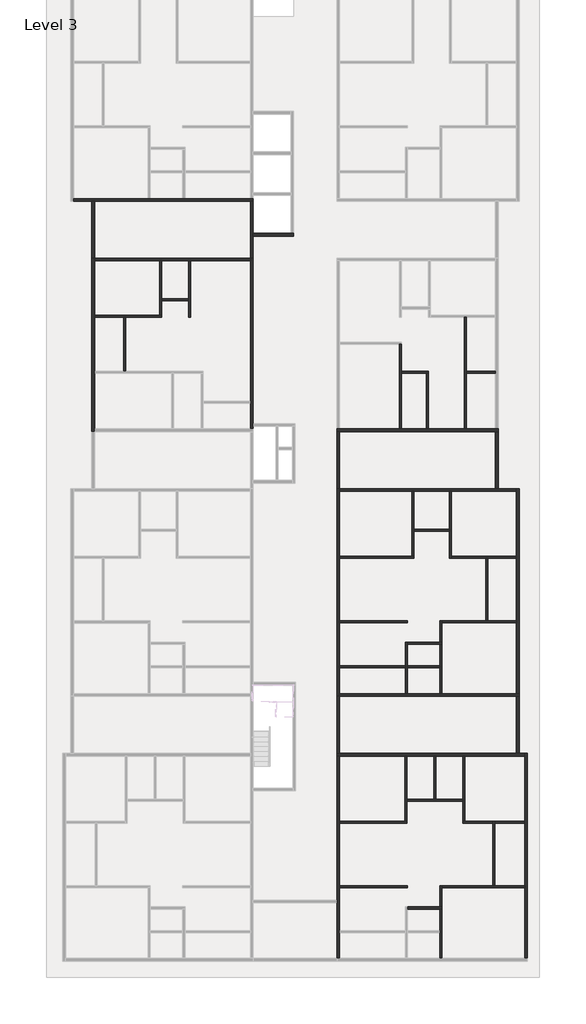
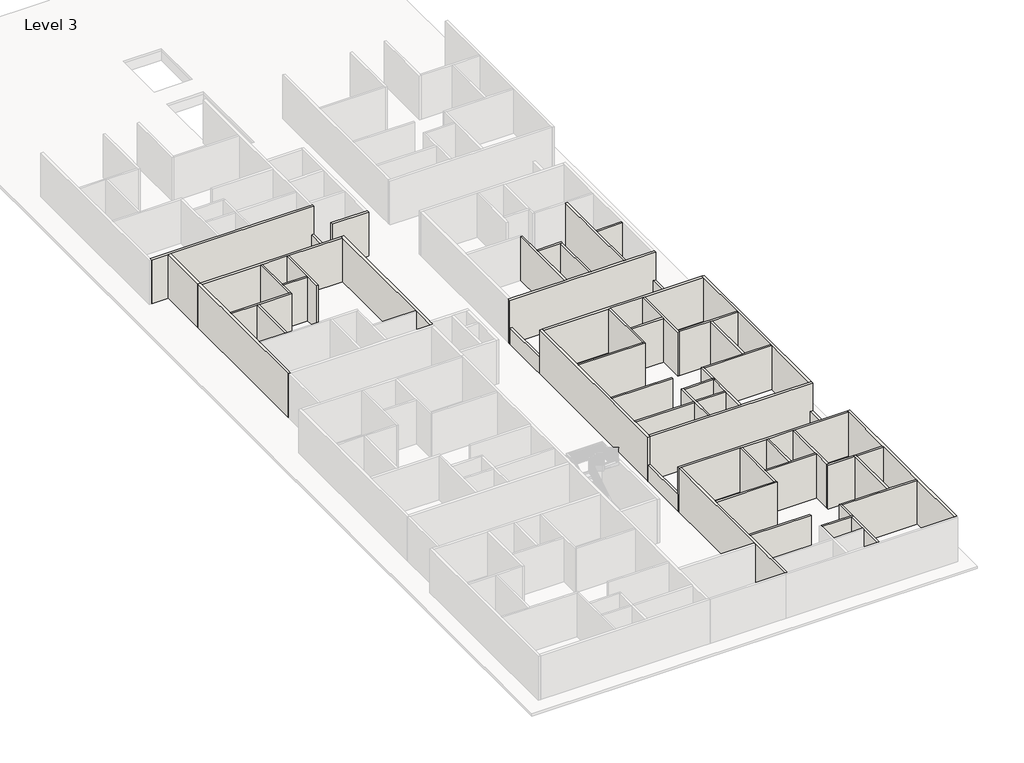
# One storey, part 2 of 8: 56 walls.
"""IFC4 building model written with IfcOpenShell, lengths in millimetres."""

from ifc_helpers import new_model, si_unit, frame, origin, place, context, project, spatial, polyline, outline, extrude, faceted_brep, element, save

model = new_model("IFC4")

# Units and contexts
model_context = context("Model", 3, world=origin())
ifc_project = project(units=[si_unit("LENGTHUNIT", "METRE", prefix="MILLI")], contexts=[model_context])

# Site, building, storey
site = spatial("IfcSite", under=ifc_project)
building = spatial("IfcBuilding", under=site)
storey = spatial("IfcBuildingStorey", under=building, Name="Level 3", Elevation=31330.6172466)

# Walls
placement = place(None, origin())
element("IfcWall", 1, ObjectType="4.5\"", at=placement, inside=storey, context=model_context, shape_type="Brep", body=[
    faceted_brep([(-12531.5544854, 2100.0216096, 31330.6172466), (-10907.2415084, 2100.0216096, 31330.6172466), (-10792.9415084, 2100.0216096, 31330.6172466), (-8759.6544854, 2100.0216096, 31330.6172466), (-8759.6544854, 2100.0216096, 34378.6172466), (-10792.9415084, 2100.0216096, 34378.6172466), (-10907.2415084, 2100.0216096, 34378.6172466), (-12531.5544854, 2100.0216096, 34378.6172466), (-12531.5544854, 2214.3216096, 31330.6172466), (-12531.5544854, 2214.3216096, 34378.6172466), (-8873.9544854, 2214.3216096, 34378.6172466), (-8759.6544854, 2214.3216096, 34378.6172466), (-8759.6544854, 2214.3216096, 31330.6172466), (-8873.9544854, 2214.3216096, 31330.6172466)], [[[0, 1, 2, 3, 4, 5, 6, 7]], [[8, 9, 10, 11, 12, 13]], [[3, 2, 1, 0, 8, 13, 12]], [[0, 7, 9, 8]], [[4, 3, 12, 11]], [[7, 6, 5, 4, 11, 10, 9]]]),
])
element("IfcWall", 2, ObjectType="4.5\"", at=placement, inside=storey, context=model_context, shape_type="Brep", body=[
    faceted_brep([(-8759.6544854, 2214.3216096, 31330.6172466), (-8759.6544854, 3014.4216096, 31330.6172466), (-8759.6544854, 3128.7216096, 31330.6172466), (-8759.6544854, 5264.2743917, 31330.6172466), (-8759.6544854, 5264.2743917, 34378.6172466), (-8759.6544854, 3128.7216096, 34378.6172466), (-8759.6544854, 3014.4216096, 34378.6172466), (-8759.6544854, 2214.3216096, 34378.6172466), (-8873.9544854, 2214.3216096, 31330.6172466), (-8873.9544854, 2214.3216096, 34378.6172466), (-8873.9544854, 5264.2743917, 34378.6172466), (-8873.9544854, 5264.2743917, 31330.6172466)], [[[0, 1, 2, 3, 4, 5, 6, 7]], [[8, 9, 10, 11]], [[3, 2, 1, 0, 8, 11]], [[0, 7, 9, 8]], [[4, 3, 11, 10]], [[7, 6, 5, 4, 10, 9]]]),
])
element("IfcWall", 3, ObjectType="4.5\"", at=placement, inside=storey, context=model_context, shape_type="Brep", body=[
    faceted_brep([(-7235.6544854, 5264.2743917, 31330.6172466), (-7235.6544854, 3128.7216096, 31330.6172466), (-7235.6544854, 3014.4216096, 31330.6172466), (-7235.6544854, 2100.0216096, 31330.6172466), (-7235.6544854, 2100.0216096, 34378.6172466), (-7235.6544854, 3014.4216096, 34378.6172466), (-7235.6544854, 3128.7216096, 34378.6172466), (-7235.6544854, 5264.2743917, 34378.6172466), (-7121.3544854, 5264.2743917, 31330.6172466), (-7121.3544854, 5264.2743917, 34378.6172466), (-7121.3544854, 2100.0216096, 34378.6172466), (-7121.3544854, 2100.0216096, 31330.6172466)], [[[0, 1, 2, 3, 4, 5, 6, 7]], [[8, 9, 10, 11]], [[3, 2, 1, 0, 8, 11]], [[4, 3, 11, 10]], [[0, 7, 9, 8]], [[7, 6, 5, 4, 10, 9]]]),
])
element("IfcWall", 4, ObjectType="4.5\"", at=placement, inside=storey, context=model_context, shape_type="SweptSolid", body=[
    extrude(outline(polyline([(-7235.6544854, 3014.4216096), (-8759.6544854, 3014.4216096), (-8759.6544854, 3128.7216096), (-7235.6544854, 3128.7216096), (-7235.6544854, 3014.4216096)])), frame((0.0, 0.0, 31330.6172466), z_axis=(0.0, 0.0, 1.0), x_axis=(1.0, 0.0, 0.0)), (0.0, 0.0, 1.0), 3048.0),
])
element("IfcWall", 5, ObjectType="4.5\"", at=placement, inside=storey, context=model_context, shape_type="SweptSolid", body=[
    extrude(outline(polyline([(-10907.2415084, -947.4344126), (-10907.2415084, 2100.0216096), (-10792.9415084, 2100.0216096), (-10792.9415084, -947.4344126), (-10907.2415084, -947.4344126)])), frame((0.0, 0.0, 31330.6172466), z_axis=(0.0, 0.0, 1.0), x_axis=(1.0, 0.0, 0.0)), (0.0, 0.0, 1.0), 3048.0),
])
element("IfcWall", 6, ObjectType="4.5\"", at=placement, inside=storey, context=model_context, shape_type="Brep", body=[
    faceted_brep([(5056.6584916, -31173.4344126, 31330.6172466), (6885.4584916, -31173.4344126, 31330.6172466), (6999.7584916, -31173.4344126, 31330.6172466), (6999.7584916, -31173.4344126, 34378.6172466), (6885.4584916, -31173.4344126, 34378.6172466), (5056.6584916, -31173.4344126, 34378.6172466), (5056.6584916, -31059.1344126, 31330.6172466), (5056.6584916, -31059.1344126, 34378.6172466), (6885.4584916, -31059.1344126, 34378.6172466), (6999.7584916, -31059.1344126, 34378.6172466), (6999.7584916, -31059.1344126, 31330.6172466), (6885.4584916, -31059.1344126, 31330.6172466)], [[[0, 1, 2, 3, 4, 5]], [[6, 7, 8, 9, 10, 11]], [[2, 1, 0, 6, 11, 10]], [[0, 5, 7, 6]], [[3, 2, 10, 9]], [[5, 4, 3, 9, 8, 7]]]),
])
element("IfcWall", 7, ObjectType="4.5\"", at=placement, inside=storey, context=model_context, shape_type="Brep", body=[
    faceted_brep([(6885.4584916, -31173.4344126, 31330.6172466), (6885.4584916, -32392.6344126, 31330.6172466), (6885.4584916, -32506.9344126, 31330.6172466), (6885.4584916, -33954.7344126, 31330.6172466), (6885.4584916, -33954.7344126, 34378.6172466), (6885.4584916, -32506.9344126, 34378.6172466), (6885.4584916, -32392.6344126, 34378.6172466), (6885.4584916, -31173.4344126, 34378.6172466), (6999.7584916, -31173.4344126, 31330.6172466), (6999.7584916, -31173.4344126, 34378.6172466), (6999.7584916, -33954.7344126, 34378.6172466), (6999.7584916, -33954.7344126, 31330.6172466)], [[[0, 1, 2, 3, 4, 5, 6, 7]], [[8, 9, 10, 11]], [[3, 2, 1, 0, 8, 11]], [[0, 7, 9, 8]], [[4, 3, 11, 10]], [[7, 6, 5, 4, 10, 9]]]),
])
element("IfcWall", 8, ObjectType="4.5\"", at=placement, inside=storey, context=model_context, shape_type="Brep", body=[
    faceted_brep([(6999.7584916, -31059.1344126, 31330.6172466), (6999.7584916, -29966.9344126, 31330.6172466), (6999.7584916, -29852.6344126, 31330.6172466), (6999.7584916, -29852.6344126, 34378.6172466), (6999.7584916, -29966.9344126, 34378.6172466), (6999.7584916, -31059.1344126, 34378.6172466), (6885.4584916, -31059.1344126, 31330.6172466), (6885.4584916, -31059.1344126, 34378.6172466), (6885.4584916, -29852.6344126, 34378.6172466), (6885.4584916, -29852.6344126, 31330.6172466)], [[[0, 1, 2, 3, 4, 5]], [[6, 7, 8, 9]], [[2, 1, 0, 6, 9]], [[0, 5, 7, 6]], [[3, 2, 9, 8]], [[5, 4, 3, 8, 7]]]),
])
element("IfcWall", 9, ObjectType="4.5\"", at=placement, inside=storey, context=model_context, shape_type="Brep", body=[
    faceted_brep([(6999.7584916, -29966.9344126, 31330.6172466), (11660.6584916, -29966.9344126, 31330.6172466), (11660.6584916, -29966.9344126, 34378.6172466), (6999.7584916, -29966.9344126, 34378.6172466), (6999.7584916, -29852.6344126, 31330.6172466), (6999.7584916, -29852.6344126, 34378.6172466), (9869.9584916, -29852.6344126, 34378.6172466), (9984.2584916, -29852.6344126, 34378.6172466), (11660.6584916, -29852.6344126, 34378.6172466), (11660.6584916, -29852.6344126, 31330.6172466), (9984.2584916, -29852.6344126, 31330.6172466), (9869.9584916, -29852.6344126, 31330.6172466)], [[[0, 1, 2, 3]], [[4, 5, 6, 7, 8, 9, 10, 11]], [[1, 0, 4, 11, 10, 9]], [[0, 3, 5, 4]], [[2, 1, 9, 8]], [[3, 2, 8, 7, 6, 5]]]),
])
element("IfcWall", 10, ObjectType="4.5\"", at=placement, inside=storey, context=model_context, shape_type="SweptSolid", body=[
    extrude(outline(polyline([(5056.6584916, -29966.9344126), (1259.3584916, -29966.9344126), (1259.3584916, -29852.6344126), (5056.6584916, -29852.6344126), (5056.6584916, -29966.9344126)])), frame((0.0, 0.0, 31330.6172466), z_axis=(0.0, 0.0, 1.0), x_axis=(1.0, 0.0, 0.0)), (0.0, 0.0, 1.0), 3048.0),
])
element("IfcWall", 11, ObjectType="4.5\"", at=placement, inside=storey, context=model_context, shape_type="Brep", body=[
    faceted_brep([(1259.3584916, -26347.4344126, 31330.6172466), (5031.2584916, -26347.4344126, 31330.6172466), (5031.2584916, -26347.4344126, 34378.6172466), (1259.3584916, -26347.4344126, 34378.6172466), (1259.3584916, -26233.1344126, 31330.6172466), (1259.3584916, -26233.1344126, 34378.6172466), (4916.9584916, -26233.1344126, 34378.6172466), (5031.2584916, -26233.1344126, 34378.6172466), (5031.2584916, -26233.1344126, 31330.6172466), (4916.9584916, -26233.1344126, 31330.6172466)], [[[0, 1, 2, 3]], [[4, 5, 6, 7, 8, 9]], [[1, 0, 4, 9, 8]], [[0, 3, 5, 4]], [[2, 1, 8, 7]], [[3, 2, 7, 6, 5]]]),
])
element("IfcWall", 12, ObjectType="4.5\"", at=placement, inside=storey, context=model_context, shape_type="Brep", body=[
    faceted_brep([(5031.2584916, -26233.1344126, 31330.6172466), (5031.2584916, -25128.2344126, 31330.6172466), (5031.2584916, -25013.9344126, 31330.6172466), (5031.2584916, -22575.5344126, 31330.6172466), (5031.2584916, -22575.5344126, 34378.6172466), (5031.2584916, -25013.9344126, 34378.6172466), (5031.2584916, -25128.2344126, 34378.6172466), (5031.2584916, -26233.1344126, 34378.6172466), (4916.9584916, -26233.1344126, 31330.6172466), (4916.9584916, -26233.1344126, 34378.6172466), (4916.9584916, -22575.5344126, 34378.6172466), (4916.9584916, -22575.5344126, 31330.6172466)], [[[0, 1, 2, 3, 4, 5, 6, 7]], [[8, 9, 10, 11]], [[3, 2, 1, 0, 8, 11]], [[0, 7, 9, 8]], [[4, 3, 11, 10]], [[7, 6, 5, 4, 10, 9]]]),
])
element("IfcWall", 13, ObjectType="4.5\"", at=placement, inside=storey, context=model_context, shape_type="Brep", body=[
    faceted_brep([(9984.2584916, -29852.6344126, 31330.6172466), (9984.2584916, -26347.4344126, 31330.6172466), (9984.2584916, -26233.1344126, 31330.6172466), (9984.2584916, -26233.1344126, 34378.6172466), (9984.2584916, -26347.4344126, 34378.6172466), (9984.2584916, -29852.6344126, 34378.6172466), (9869.9584916, -29852.6344126, 31330.6172466), (9869.9584916, -29852.6344126, 34378.6172466), (9869.9584916, -26347.4344126, 34378.6172466), (9869.9584916, -26233.1344126, 34378.6172466), (9869.9584916, -26233.1344126, 31330.6172466), (9869.9584916, -26347.4344126, 31330.6172466)], [[[0, 1, 2, 3, 4, 5]], [[6, 7, 8, 9, 10, 11]], [[2, 1, 0, 6, 11, 10]], [[0, 5, 7, 6]], [[3, 2, 10, 9]], [[5, 4, 3, 9, 8, 7]]]),
])
element("IfcWall", 14, ObjectType="4.5\"", at=placement, inside=storey, context=model_context, shape_type="SweptSolid", body=[
    extrude(outline(polyline([(11660.6584916, -26347.4344126), (9984.2584916, -26347.4344126), (9984.2584916, -26233.1344126), (11660.6584916, -26233.1344126), (11660.6584916, -26347.4344126)])), frame((0.0, 0.0, 31330.6172466), z_axis=(0.0, 0.0, 1.0), x_axis=(1.0, 0.0, 0.0)), (0.0, 0.0, 1.0), 3048.0),
])
element("IfcWall", 15, ObjectType="4.5\"", at=placement, inside=storey, context=model_context, shape_type="Brep", body=[
    faceted_brep([(9869.9584916, -26233.1344126, 31330.6172466), (8307.8584916, -26233.1344126, 31330.6172466), (8193.5584916, -26233.1344126, 31330.6172466), (8193.5584916, -26233.1344126, 34378.6172466), (8307.8584916, -26233.1344126, 34378.6172466), (9869.9584916, -26233.1344126, 34378.6172466), (9869.9584916, -26347.4344126, 31330.6172466), (9869.9584916, -26347.4344126, 34378.6172466), (8193.5584916, -26347.4344126, 34378.6172466), (8193.5584916, -26347.4344126, 31330.6172466)], [[[0, 1, 2, 3, 4, 5]], [[6, 7, 8, 9]], [[2, 1, 0, 6, 9]], [[0, 5, 7, 6]], [[3, 2, 9, 8]], [[5, 4, 3, 8, 7]]]),
])
element("IfcWall", 16, ObjectType="4.5\"", at=placement, inside=storey, context=model_context, shape_type="Brep", body=[
    faceted_brep([(8307.8584916, -26233.1344126, 31330.6172466), (8307.8584916, -22575.5344126, 31330.6172466), (8307.8584916, -22575.5344126, 34378.6172466), (8307.8584916, -26233.1344126, 34378.6172466), (8193.5584916, -26233.1344126, 31330.6172466), (8193.5584916, -26233.1344126, 34378.6172466), (8193.5584916, -25128.2344126, 34378.6172466), (8193.5584916, -25013.9344126, 34378.6172466), (8193.5584916, -22575.5344126, 34378.6172466), (8193.5584916, -22575.5344126, 31330.6172466), (8193.5584916, -25013.9344126, 31330.6172466), (8193.5584916, -25128.2344126, 31330.6172466)], [[[0, 1, 2, 3]], [[4, 5, 6, 7, 8, 9, 10, 11]], [[1, 0, 4, 11, 10, 9]], [[0, 3, 5, 4]], [[2, 1, 9, 8]], [[3, 2, 8, 7, 6, 5]]]),
])
element("IfcWall", 17, ObjectType="4.5\"", at=placement, inside=storey, context=model_context, shape_type="Brep", body=[
    faceted_brep([(5031.2584916, -25128.2344126, 31330.6172466), (8193.5584916, -25128.2344126, 31330.6172466), (8193.5584916, -25128.2344126, 34378.6172466), (5031.2584916, -25128.2344126, 34378.6172466), (5031.2584916, -25013.9344126, 31330.6172466), (5031.2584916, -25013.9344126, 34378.6172466), (6555.2584916, -25013.9344126, 34378.6172466), (6669.5584916, -25013.9344126, 34378.6172466), (8193.5584916, -25013.9344126, 34378.6172466), (8193.5584916, -25013.9344126, 31330.6172466), (6669.5584916, -25013.9344126, 31330.6172466), (6555.2584916, -25013.9344126, 31330.6172466)], [[[0, 1, 2, 3]], [[4, 5, 6, 7, 8, 9, 10, 11]], [[1, 0, 4, 11, 10, 9]], [[0, 3, 5, 4]], [[2, 1, 9, 8]], [[3, 2, 8, 7, 6, 5]]]),
])
element("IfcWall", 18, ObjectType="4.5\"", at=placement, inside=storey, context=model_context, shape_type="SweptSolid", body=[
    extrude(outline(polyline([(6555.2584916, -25013.9344126), (6555.2584916, -22575.5344126), (6669.5584916, -22575.5344126), (6669.5584916, -25013.9344126), (6555.2584916, -25013.9344126)])), frame((0.0, 0.0, 31330.6172466), z_axis=(0.0, 0.0, 1.0), x_axis=(1.0, 0.0, 0.0)), (0.0, 0.0, 1.0), 3048.0),
])
element("IfcWall", 19, ObjectType="4.5\"", at=placement, inside=storey, context=model_context, shape_type="SweptSolid", body=[
    extrude(outline(polyline([(4942.3584916, -17622.5344126), (1259.3584916, -17622.5344126), (1259.3584916, -17508.2344126), (4942.3584916, -17508.2344126), (4942.3584916, -17622.5344126)])), frame((0.0, 0.0, 31330.6172466), z_axis=(0.0, 0.0, 1.0), x_axis=(1.0, 0.0, 0.0)), (0.0, 0.0, 1.0), 3048.0),
])
element("IfcWall", 20, ObjectType="4.5\"", at=placement, inside=storey, context=model_context, shape_type="Brep", body=[
    faceted_brep([(4942.3584916, -16174.7344126, 31330.6172466), (4942.3584916, -17508.2344126, 31330.6172466), (4942.3584916, -17622.5344126, 31330.6172466), (4942.3584916, -19070.3344126, 31330.6172466), (4942.3584916, -19070.3344126, 34378.6172466), (4942.3584916, -17622.5344126, 34378.6172466), (4942.3584916, -17508.2344126, 34378.6172466), (4942.3584916, -16174.7344126, 34378.6172466), (5056.6584916, -16174.7344126, 31330.6172466), (5056.6584916, -16174.7344126, 34378.6172466), (5056.6584916, -16289.0344126, 34378.6172466), (5056.6584916, -17508.2344126, 34378.6172466), (5056.6584916, -17622.5344126, 34378.6172466), (5056.6584916, -19070.3344126, 34378.6172466), (5056.6584916, -19070.3344126, 31330.6172466), (5056.6584916, -17622.5344126, 31330.6172466), (5056.6584916, -17508.2344126, 31330.6172466), (5056.6584916, -16289.0344126, 31330.6172466)], [[[0, 1, 2, 3, 4, 5, 6, 7]], [[8, 9, 10, 11, 12, 13, 14, 15, 16, 17]], [[3, 2, 1, 0, 8, 17, 16, 15, 14]], [[4, 3, 14, 13]], [[0, 7, 9, 8]], [[7, 6, 5, 4, 13, 12, 11, 10, 9]]]),
])
element("IfcWall", 21, ObjectType="4.5\"", at=placement, inside=storey, context=model_context, shape_type="Brep", body=[
    faceted_brep([(5056.6584916, -16289.0344126, 31330.6172466), (6885.4584916, -16289.0344126, 31330.6172466), (6999.7584916, -16289.0344126, 31330.6172466), (6999.7584916, -16289.0344126, 34378.6172466), (6885.4584916, -16289.0344126, 34378.6172466), (5056.6584916, -16289.0344126, 34378.6172466), (5056.6584916, -16174.7344126, 31330.6172466), (5056.6584916, -16174.7344126, 34378.6172466), (6885.4584916, -16174.7344126, 34378.6172466), (6999.7584916, -16174.7344126, 34378.6172466), (6999.7584916, -16174.7344126, 31330.6172466), (6885.4584916, -16174.7344126, 31330.6172466)], [[[0, 1, 2, 3, 4, 5]], [[6, 7, 8, 9, 10, 11]], [[2, 1, 0, 6, 11, 10]], [[0, 5, 7, 6]], [[3, 2, 10, 9]], [[5, 4, 3, 9, 8, 7]]]),
])
element("IfcWall", 22, ObjectType="4.5\"", at=placement, inside=storey, context=model_context, shape_type="Brep", body=[
    faceted_brep([(6885.4584916, -16289.0344126, 31330.6172466), (6885.4584916, -17508.2344126, 31330.6172466), (6885.4584916, -17622.5344126, 31330.6172466), (6885.4584916, -19070.3344126, 31330.6172466), (6885.4584916, -19070.3344126, 34378.6172466), (6885.4584916, -17622.5344126, 34378.6172466), (6885.4584916, -17508.2344126, 34378.6172466), (6885.4584916, -16289.0344126, 34378.6172466), (6999.7584916, -16289.0344126, 31330.6172466), (6999.7584916, -16289.0344126, 34378.6172466), (6999.7584916, -19070.3344126, 34378.6172466), (6999.7584916, -19070.3344126, 31330.6172466)], [[[0, 1, 2, 3, 4, 5, 6, 7]], [[8, 9, 10, 11]], [[3, 2, 1, 0, 8, 11]], [[0, 7, 9, 8]], [[4, 3, 11, 10]], [[7, 6, 5, 4, 10, 9]]]),
])
element("IfcWall", 23, ObjectType="4.5\"", at=placement, inside=storey, context=model_context, shape_type="SweptSolid", body=[
    extrude(outline(polyline([(6885.4584916, -17622.5344126), (5056.6584916, -17622.5344126), (5056.6584916, -17508.2344126), (6885.4584916, -17508.2344126), (6885.4584916, -17622.5344126)])), frame((0.0, 0.0, 31330.6172466), z_axis=(0.0, 0.0, 1.0), x_axis=(1.0, 0.0, 0.0)), (0.0, 0.0, 1.0), 3048.0),
])
element("IfcWall", 24, ObjectType="4.5\"", at=placement, inside=storey, context=model_context, shape_type="Brep", body=[
    faceted_brep([(6999.7584916, -16174.7344126, 31330.6172466), (6999.7584916, -15082.5344126, 31330.6172466), (6999.7584916, -14968.2344126, 31330.6172466), (6999.7584916, -14968.2344126, 34378.6172466), (6999.7584916, -15082.5344126, 34378.6172466), (6999.7584916, -16174.7344126, 34378.6172466), (6885.4584916, -16174.7344126, 31330.6172466), (6885.4584916, -16174.7344126, 34378.6172466), (6885.4584916, -14968.2344126, 34378.6172466), (6885.4584916, -14968.2344126, 31330.6172466)], [[[0, 1, 2, 3, 4, 5]], [[6, 7, 8, 9]], [[2, 1, 0, 6, 9]], [[0, 5, 7, 6]], [[3, 2, 9, 8]], [[5, 4, 3, 8, 7]]]),
])
element("IfcWall", 25, ObjectType="4.5\"", at=placement, inside=storey, context=model_context, shape_type="Brep", body=[
    faceted_brep([(6999.7584916, -15082.5344126, 31330.6172466), (11208.5214687, -15082.5344126, 31330.6172466), (11208.5214687, -15082.5344126, 34378.6172466), (6999.7584916, -15082.5344126, 34378.6172466), (6999.7584916, -14968.2344126, 31330.6172466), (6999.7584916, -14968.2344126, 34378.6172466), (9469.9084916, -14968.2344126, 34378.6172466), (9584.2084916, -14968.2344126, 34378.6172466), (11208.5214687, -14968.2344126, 34378.6172466), (11208.5214687, -14968.2344126, 31330.6172466), (9584.2084916, -14968.2344126, 31330.6172466), (9469.9084916, -14968.2344126, 31330.6172466)], [[[0, 1, 2, 3]], [[4, 5, 6, 7, 8, 9, 10, 11]], [[1, 0, 4, 11, 10, 9]], [[0, 3, 5, 4]], [[2, 1, 9, 8]], [[3, 2, 8, 7, 6, 5]]]),
])
element("IfcWall", 26, ObjectType="4.5\"", at=placement, inside=storey, context=model_context, shape_type="SweptSolid", body=[
    extrude(outline(polyline([(5056.6584916, -15082.5344126), (1259.3584916, -15082.5344126), (1259.3584916, -14968.2344126), (5056.6584916, -14968.2344126), (5056.6584916, -15082.5344126)])), frame((0.0, 0.0, 31330.6172466), z_axis=(0.0, 0.0, 1.0), x_axis=(1.0, 0.0, 0.0)), (0.0, 0.0, 1.0), 3048.0),
])
element("IfcWall", 27, ObjectType="4.5\"", at=placement, inside=storey, context=model_context, shape_type="Brep", body=[
    faceted_brep([(1259.3584916, -11463.0344126, 31330.6172466), (5430.0214687, -11463.0344126, 31330.6172466), (5430.0214687, -11463.0344126, 34378.6172466), (1259.3584916, -11463.0344126, 34378.6172466), (1259.3584916, -11348.7344126, 31330.6172466), (1259.3584916, -11348.7344126, 34378.6172466), (5315.7214687, -11348.7344126, 34378.6172466), (5430.0214687, -11348.7344126, 34378.6172466), (5430.0214687, -11348.7344126, 31330.6172466), (5315.7214687, -11348.7344126, 31330.6172466)], [[[0, 1, 2, 3]], [[4, 5, 6, 7, 8, 9]], [[1, 0, 4, 9, 8]], [[0, 3, 5, 4]], [[2, 1, 8, 7]], [[3, 2, 7, 6, 5]]]),
])
element("IfcWall", 28, ObjectType="4.5\"", at=placement, inside=storey, context=model_context, shape_type="Brep", body=[
    faceted_brep([(5430.0214687, -11348.7344126, 31330.6172466), (5430.0214687, -9939.0344126, 31330.6172466), (5430.0214687, -9824.7344126, 31330.6172466), (5430.0214687, -7691.1344126, 31330.6172466), (5430.0214687, -7691.1344126, 34378.6172466), (5430.0214687, -9824.7344126, 34378.6172466), (5430.0214687, -9939.0344126, 34378.6172466), (5430.0214687, -11348.7344126, 34378.6172466), (5315.7214687, -11348.7344126, 31330.6172466), (5315.7214687, -11348.7344126, 34378.6172466), (5315.7214687, -7691.1344126, 34378.6172466), (5315.7214687, -7691.1344126, 31330.6172466)], [[[0, 1, 2, 3, 4, 5, 6, 7]], [[8, 9, 10, 11]], [[3, 2, 1, 0, 8, 11]], [[0, 7, 9, 8]], [[4, 3, 11, 10]], [[7, 6, 5, 4, 10, 9]]]),
])
element("IfcWall", 29, ObjectType="4.5\"", at=placement, inside=storey, context=model_context, shape_type="SweptSolid", body=[
    extrude(outline(polyline([(7436.6214687, -9939.0344126), (5430.0214687, -9939.0344126), (5430.0214687, -9824.7344126), (7436.6214687, -9824.7344126), (7436.6214687, -9939.0344126)])), frame((0.0, 0.0, 31330.6172466), z_axis=(0.0, 0.0, 1.0), x_axis=(1.0, 0.0, 0.0)), (0.0, 0.0, 1.0), 3048.0),
])
element("IfcWall", 30, ObjectType="4.5\"", at=placement, inside=storey, context=model_context, shape_type="Brep", body=[
    faceted_brep([(7436.6214687, -7691.1344126, 31330.6172466), (7436.6214687, -9824.7344126, 31330.6172466), (7436.6214687, -9939.0344126, 31330.6172466), (7436.6214687, -11463.0344126, 31330.6172466), (7436.6214687, -11463.0344126, 34378.6172466), (7436.6214687, -9939.0344126, 34378.6172466), (7436.6214687, -9824.7344126, 34378.6172466), (7436.6214687, -7691.1344126, 34378.6172466), (7550.9214687, -7691.1344126, 31330.6172466), (7550.9214687, -7691.1344126, 34378.6172466), (7550.9214687, -11348.7344126, 34378.6172466), (7550.9214687, -11463.0344126, 34378.6172466), (7550.9214687, -11463.0344126, 31330.6172466), (7550.9214687, -11348.7344126, 31330.6172466)], [[[0, 1, 2, 3, 4, 5, 6, 7]], [[8, 9, 10, 11, 12, 13]], [[3, 2, 1, 0, 8, 13, 12]], [[0, 7, 9, 8]], [[4, 3, 12, 11]], [[7, 6, 5, 4, 11, 10, 9]]]),
])
element("IfcWall", 31, ObjectType="4.5\"", at=placement, inside=storey, context=model_context, shape_type="Brep", body=[
    faceted_brep([(7550.9214687, -11463.0344126, 31330.6172466), (9469.9084916, -11463.0344126, 31330.6172466), (9584.2084916, -11463.0344126, 31330.6172466), (11208.5214687, -11463.0344126, 31330.6172466), (11208.5214687, -11463.0344126, 34378.6172466), (9584.2084916, -11463.0344126, 34378.6172466), (9469.9084916, -11463.0344126, 34378.6172466), (7550.9214687, -11463.0344126, 34378.6172466), (7550.9214687, -11348.7344126, 31330.6172466), (7550.9214687, -11348.7344126, 34378.6172466), (11208.5214687, -11348.7344126, 34378.6172466), (11208.5214687, -11348.7344126, 31330.6172466)], [[[0, 1, 2, 3, 4, 5, 6, 7]], [[8, 9, 10, 11]], [[3, 2, 1, 0, 8, 11]], [[0, 7, 9, 8]], [[4, 3, 11, 10]], [[7, 6, 5, 4, 10, 9]]]),
])
element("IfcWall", 32, ObjectType="4.5\"", at=placement, inside=storey, context=model_context, shape_type="SweptSolid", body=[
    extrude(outline(polyline([(9469.9084916, -14968.2344126), (9469.9084916, -11463.0344126), (9584.2084916, -11463.0344126), (9584.2084916, -14968.2344126), (9469.9084916, -14968.2344126)])), frame((0.0, 0.0, 31330.6172466), z_axis=(0.0, 0.0, 1.0), x_axis=(1.0, 0.0, 0.0)), (0.0, 0.0, 1.0), 3048.0),
])
element("IfcWall", 33, ObjectType="4.5\"", at=placement, inside=storey, context=model_context, shape_type="Brep", body=[
    faceted_brep([(4610.8714687, 572.7745083, 31330.6172466), (4610.8714687, -4185.9344126, 31330.6172466), (4610.8714687, -4185.9344126, 34378.6172466), (4610.8714687, 572.7745083, 34378.6172466), (4725.1714687, 572.7745083, 31330.6172466), (4725.1714687, 572.7745083, 34378.6172466), (4725.1714687, -947.4344126, 34378.6172466), (4725.1714687, -1061.7344126, 34378.6172466), (4725.1714687, -4185.9344126, 34378.6172466), (4725.1714687, -4185.9344126, 31330.6172466), (4725.1714687, -1061.7344126, 31330.6172466), (4725.1714687, -947.4344126, 31330.6172466)], [[[0, 1, 2, 3]], [[4, 5, 6, 7, 8, 9, 10, 11]], [[1, 0, 4, 11, 10, 9]], [[0, 3, 5, 4]], [[2, 1, 9, 8]], [[3, 2, 8, 7, 6, 5]]]),
])
element("IfcWall", 34, ObjectType="4.5\"", at=placement, inside=storey, context=model_context, shape_type="Brep", body=[
    faceted_brep([(4725.1714687, -1061.7344126, 31330.6172466), (6134.8714687, -1061.7344126, 31330.6172466), (6249.1714687, -1061.7344126, 31330.6172466), (6249.1714687, -1061.7344126, 34378.6172466), (6134.8714687, -1061.7344126, 34378.6172466), (4725.1714687, -1061.7344126, 34378.6172466), (4725.1714687, -947.4344126, 31330.6172466), (4725.1714687, -947.4344126, 34378.6172466), (6249.1714687, -947.4344126, 34378.6172466), (6249.1714687, -947.4344126, 31330.6172466)], [[[0, 1, 2, 3, 4, 5]], [[6, 7, 8, 9]], [[2, 1, 0, 6, 9]], [[0, 5, 7, 6]], [[3, 2, 9, 8]], [[5, 4, 3, 8, 7]]]),
])
element("IfcWall", 35, ObjectType="4.5\"", at=placement, inside=storey, context=model_context, shape_type="SweptSolid", body=[
    extrude(outline(polyline([(6134.8714687, -4185.9344126), (6134.8714687, -1061.7344126), (6249.1714687, -1061.7344126), (6249.1714687, -4185.9344126), (6134.8714687, -4185.9344126)])), frame((0.0, 0.0, 31330.6172466), z_axis=(0.0, 0.0, 1.0), x_axis=(1.0, 0.0, 0.0)), (0.0, 0.0, 1.0), 3048.0),
])
element("IfcWall", 36, ObjectType="4.5\"", at=placement, inside=storey, context=model_context, shape_type="Brep", body=[
    faceted_brep([(8396.7584916, -4185.9344126, 31330.6172466), (8396.7584916, -1061.7344126, 31330.6172466), (8396.7584916, -947.4344126, 31330.6172466), (8396.7584916, 2100.0216096, 31330.6172466), (8396.7584916, 2100.0216096, 34378.6172466), (8396.7584916, -947.4344126, 34378.6172466), (8396.7584916, -1061.7344126, 34378.6172466), (8396.7584916, -4185.9344126, 34378.6172466), (8282.4584916, -4185.9344126, 31330.6172466), (8282.4584916, -4185.9344126, 34378.6172466), (8282.4584916, 2100.0216096, 34378.6172466), (8282.4584916, 2100.0216096, 31330.6172466)], [[[0, 1, 2, 3, 4, 5, 6, 7]], [[8, 9, 10, 11]], [[3, 2, 1, 0, 8, 11]], [[0, 7, 9, 8]], [[4, 3, 11, 10]], [[7, 6, 5, 4, 10, 9]]]),
])
element("IfcWall", 37, ObjectType="4.5\"", at=placement, inside=storey, context=model_context, shape_type="SweptSolid", body=[
    extrude(outline(polyline([(8396.7584916, -947.4344126), (10021.0714687, -947.4344126), (10021.0714687, -1061.7344126), (8396.7584916, -1061.7344126), (8396.7584916, -947.4344126)])), frame((0.0, 0.0, 31330.6172466), z_axis=(0.0, 0.0, 1.0), x_axis=(1.0, 0.0, 0.0)), (0.0, 0.0, 1.0), 3048.0),
])
element("IfcWall", 38, ObjectType="6\"", at=placement, inside=storey, context=model_context, shape_type="Brep", body=[
    faceted_brep([(-13719.0044854, 8615.1216096, 31330.6172466), (-12683.9544854, 8615.1216096, 31330.6172466), (-12531.5544854, 8615.1216096, 31330.6172466), (-3769.8415084, 8615.1216096, 31330.6172466), (-3617.4415084, 8615.1216096, 31330.6172466), (-3617.4415084, 8615.1216096, 32549.8172466), (-3617.4415084, 8615.1216096, 34378.6172466), (-12531.5544854, 8615.1216096, 34378.6172466), (-12683.9544854, 8615.1216096, 34378.6172466), (-13719.0044854, 8615.1216096, 34378.6172466), (-13719.0044854, 8767.5216096, 31330.6172466), (-13719.0044854, 8767.5216096, 34378.6172466), (-9510.2415084, 8767.5216096, 34378.6172466), (-9395.9415084, 8767.5216096, 34378.6172466), (-7567.1415084, 8767.5216096, 34378.6172466), (-7452.8415084, 8767.5216096, 34378.6172466), (-3769.8415084, 8767.5216096, 34378.6172466), (-3617.4415084, 8767.5216096, 34378.6172466), (-3617.4415084, 8767.5216096, 31330.6172466), (-3769.8415084, 8767.5216096, 31330.6172466), (-7452.8415084, 8767.5216096, 31330.6172466), (-7567.1415084, 8767.5216096, 31330.6172466), (-9395.9415084, 8767.5216096, 31330.6172466), (-9510.2415084, 8767.5216096, 31330.6172466)], [[[0, 1, 2, 3, 4, 5, 6, 7, 8, 9]], [[10, 11, 12, 13, 14, 15, 16, 17, 18, 19, 20, 21, 22, 23]], [[4, 3, 2, 1, 0, 10, 23, 22, 21, 20, 19, 18]], [[0, 9, 11, 10]], [[4, 18, 17, 6, 5]], [[9, 8, 7, 6, 17, 16, 15, 14, 13, 12, 11]]]),
])
element("IfcWall", 39, ObjectType="6\"", at=placement, inside=storey, context=model_context, shape_type="Brep", body=[
    faceted_brep([(-12683.9544854, 5416.6743917, 31330.6172466), (-12683.9544854, -4338.3344126, 31330.6172466), (-12683.9544854, -4338.3344126, 34378.6172466), (-12683.9544854, 5416.6743917, 34378.6172466), (-12531.5544854, 5416.6743917, 31330.6172466), (-12531.5544854, 5416.6743917, 34378.6172466), (-12531.5544854, 5264.2743917, 34378.6172466), (-12531.5544854, 2214.3216096, 34378.6172466), (-12531.5544854, 2100.0216096, 34378.6172466), (-12531.5544854, -947.4344126, 34378.6172466), (-12531.5544854, -1061.7344126, 34378.6172466), (-12531.5544854, -4185.9344126, 34378.6172466), (-12531.5544854, -4338.3344126, 34378.6172466), (-12531.5544854, -4338.3344126, 31330.6172466), (-12531.5544854, -4185.9344126, 31330.6172466), (-12531.5544854, -1061.7344126, 31330.6172466), (-12531.5544854, -947.4344126, 31330.6172466), (-12531.5544854, 2100.0216096, 31330.6172466), (-12531.5544854, 2214.3216096, 31330.6172466), (-12531.5544854, 5264.2743917, 31330.6172466)], [[[0, 1, 2, 3]], [[4, 5, 6, 7, 8, 9, 10, 11, 12, 13, 14, 15, 16, 17, 18, 19]], [[1, 0, 4, 19, 18, 17, 16, 15, 14, 13]], [[2, 1, 13, 12]], [[0, 3, 5, 4]], [[3, 2, 12, 11, 10, 9, 8, 7, 6, 5]]]),
])
element("IfcWall", 40, ObjectType="6\"", at=placement, inside=storey, context=model_context, shape_type="Brep", body=[
    faceted_brep([(-3617.4415084, -4185.9344126, 31330.6172466), (-3617.4415084, -4034.6751812, 31330.6172466), (-3617.4415084, -3882.2751812, 31330.6172466), (-3617.4415084, 5416.6743917, 31330.6172466), (-3617.4415084, 5416.6743917, 34378.6172466), (-3617.4415084, -3882.2751812, 34378.6172466), (-3617.4415084, -4034.6751812, 34378.6172466), (-3617.4415084, -4185.9344126, 34378.6172466), (-3769.8415084, -4185.9344126, 31330.6172466), (-3769.8415084, -4185.9344126, 34378.6172466), (-3769.8415084, -2738.1344126, 34378.6172466), (-3769.8415084, -2623.8344126, 34378.6172466), (-3769.8415084, 5264.2743917, 34378.6172466), (-3769.8415084, 5416.6743917, 34378.6172466), (-3769.8415084, 5416.6743917, 31330.6172466), (-3769.8415084, 5264.2743917, 31330.6172466), (-3769.8415084, -2623.8344126, 31330.6172466), (-3769.8415084, -2738.1344126, 31330.6172466)], [[[0, 1, 2, 3, 4, 5, 6, 7]], [[8, 9, 10, 11, 12, 13, 14, 15, 16, 17]], [[3, 2, 1, 0, 8, 17, 16, 15, 14]], [[0, 7, 9, 8]], [[3, 14, 13, 4]], [[7, 6, 5, 4, 13, 12, 11, 10, 9]]]),
])
element("IfcWall", 41, ObjectType="6\"", at=placement, inside=storey, context=model_context, shape_type="Brep", body=[
    faceted_brep([(-3769.8415084, 5416.6743917, 34378.6172466), (-3769.8415084, 5416.6743917, 31330.6172466), (-12531.5544854, 5416.6743917, 31330.6172466), (-12531.5544854, 5416.6743917, 34378.6172466), (-3769.8415084, 5264.2743917, 31330.6172466), (-3769.8415084, 5264.2743917, 34378.6172466), (-7121.3544854, 5264.2743917, 34378.6172466), (-7235.6544854, 5264.2743917, 34378.6172466), (-8759.6544854, 5264.2743917, 34378.6172466), (-8873.9544854, 5264.2743917, 34378.6172466), (-12531.5544854, 5264.2743917, 34378.6172466), (-12531.5544854, 5264.2743917, 31330.6172466), (-8873.9544854, 5264.2743917, 31330.6172466), (-8759.6544854, 5264.2743917, 31330.6172466), (-7235.6544854, 5264.2743917, 31330.6172466), (-7121.3544854, 5264.2743917, 31330.6172466)], [[[0, 1, 2, 3]], [[4, 5, 6, 7, 8, 9, 10, 11, 12, 13, 14, 15]], [[2, 1, 4, 15, 14, 13, 12, 11]], [[3, 2, 11, 10]], [[0, 5, 4, 1]], [[0, 3, 10, 9, 8, 7, 6, 5]]]),
])
element("IfcWall", 42, ObjectType="6\"", at=placement, inside=storey, context=model_context, shape_type="Brep", body=[
    faceted_brep([(11813.0584916, -33954.7344126, 31330.6172466), (11813.0584916, -22423.1344126, 31330.6172466), (11813.0584916, -22423.1344126, 34378.6172466), (11813.0584916, -33954.7344126, 34378.6172466), (11660.6584916, -33954.7344126, 31330.6172466), (11660.6584916, -33954.7344126, 34378.6172466), (11660.6584916, -29966.9344126, 34378.6172466), (11660.6584916, -29852.6344126, 34378.6172466), (11660.6584916, -26347.4344126, 34378.6172466), (11660.6584916, -26233.1344126, 34378.6172466), (11660.6584916, -22575.5344126, 34378.6172466), (11660.6584916, -22423.1344126, 34378.6172466), (11660.6584916, -22423.1344126, 31330.6172466), (11660.6584916, -22575.5344126, 31330.6172466), (11660.6584916, -26233.1344126, 31330.6172466), (11660.6584916, -26347.4344126, 31330.6172466), (11660.6584916, -29852.6344126, 31330.6172466), (11660.6584916, -29966.9344126, 31330.6172466)], [[[0, 1, 2, 3]], [[4, 5, 6, 7, 8, 9, 10, 11, 12, 13, 14, 15, 16, 17]], [[1, 0, 4, 17, 16, 15, 14, 13, 12]], [[0, 3, 5, 4]], [[2, 1, 12, 11]], [[3, 2, 11, 10, 9, 8, 7, 6, 5]]]),
])
element("IfcWall", 43, ObjectType="6\"", at=placement, inside=storey, context=model_context, shape_type="Brep", body=[
    faceted_brep([(11660.6584916, -22423.1344126, 31330.6172466), (11360.9214687, -22423.1344126, 31330.6172466), (11208.5214687, -22423.1344126, 31330.6172466), (1259.3584916, -22423.1344126, 31330.6172466), (1106.9584916, -22423.1344126, 31330.6172466), (1106.9584916, -22423.1344126, 32549.8172466), (1106.9584916, -22423.1344126, 34378.6172466), (11660.6584916, -22423.1344126, 34378.6172466), (11660.6584916, -22575.5344126, 31330.6172466), (11660.6584916, -22575.5344126, 34378.6172466), (8307.8584916, -22575.5344126, 34378.6172466), (8193.5584916, -22575.5344126, 34378.6172466), (6669.5584916, -22575.5344126, 34378.6172466), (6555.2584916, -22575.5344126, 34378.6172466), (5031.2584916, -22575.5344126, 34378.6172466), (4916.9584916, -22575.5344126, 34378.6172466), (1259.3584916, -22575.5344126, 34378.6172466), (1106.9584916, -22575.5344126, 34378.6172466), (1106.9584916, -22575.5344126, 31330.6172466), (1259.3584916, -22575.5344126, 31330.6172466), (4916.9584916, -22575.5344126, 31330.6172466), (5031.2584916, -22575.5344126, 31330.6172466), (6555.2584916, -22575.5344126, 31330.6172466), (6669.5584916, -22575.5344126, 31330.6172466), (8193.5584916, -22575.5344126, 31330.6172466), (8307.8584916, -22575.5344126, 31330.6172466)], [[[0, 1, 2, 3, 4, 5, 6, 7]], [[8, 9, 10, 11, 12, 13, 14, 15, 16, 17, 18, 19, 20, 21, 22, 23, 24, 25]], [[4, 3, 2, 1, 0, 8, 25, 24, 23, 22, 21, 20, 19, 18]], [[0, 7, 9, 8]], [[4, 18, 17, 6, 5]], [[7, 6, 17, 16, 15, 14, 13, 12, 11, 10, 9]]]),
])
element("IfcWall", 44, ObjectType="6\"", at=placement, inside=storey, context=model_context, shape_type="Brep", body=[
    faceted_brep([(1106.9584916, -22575.5344126, 34378.6172466), (1106.9584916, -22575.5344126, 31330.6172466), (1106.9584916, -30668.5325185, 31330.6172466), (1106.9584916, -30820.9325185, 31330.6172466), (1106.9584916, -33954.7344126, 31330.6172466), (1106.9584916, -33954.7344126, 34378.6172466), (1106.9584916, -30820.9325185, 34378.6172466), (1106.9584916, -30668.5325185, 34378.6172466), (1259.3584916, -22575.5344126, 31330.6172466), (1259.3584916, -22575.5344126, 34378.6172466), (1259.3584916, -26233.1344126, 34378.6172466), (1259.3584916, -26347.4344126, 34378.6172466), (1259.3584916, -29852.6344126, 34378.6172466), (1259.3584916, -29966.9344126, 34378.6172466), (1259.3584916, -32392.6344126, 34378.6172466), (1259.3584916, -32506.9344126, 34378.6172466), (1259.3584916, -33954.7344126, 34378.6172466), (1259.3584916, -33954.7344126, 31330.6172466), (1259.3584916, -32506.9344126, 31330.6172466), (1259.3584916, -32392.6344126, 31330.6172466), (1259.3584916, -29966.9344126, 31330.6172466), (1259.3584916, -29852.6344126, 31330.6172466), (1259.3584916, -26347.4344126, 31330.6172466), (1259.3584916, -26233.1344126, 31330.6172466)], [[[0, 1, 2, 3, 4, 5, 6, 7]], [[8, 9, 10, 11, 12, 13, 14, 15, 16, 17, 18, 19, 20, 21, 22, 23]], [[4, 3, 2, 1, 8, 23, 22, 21, 20, 19, 18, 17]], [[5, 4, 17, 16]], [[0, 9, 8, 1]], [[0, 7, 6, 5, 16, 15, 14, 13, 12, 11, 10, 9]]]),
])
element("IfcWall", 45, ObjectType="6\"", at=placement, inside=storey, context=model_context, shape_type="Brep", body=[
    faceted_brep([(1106.9584916, -7538.7344126, 34378.6172466), (1106.9584916, -7538.7344126, 31330.6172466), (1106.9584916, -19222.7344126, 31330.6172466), (1106.9584916, -19222.7344126, 34378.6172466), (1259.3584916, -7538.7344126, 31330.6172466), (1259.3584916, -7538.7344126, 34378.6172466), (1259.3584916, -7691.1344126, 34378.6172466), (1259.3584916, -11348.7344126, 34378.6172466), (1259.3584916, -11463.0344126, 34378.6172466), (1259.3584916, -14968.2344126, 34378.6172466), (1259.3584916, -15082.5344126, 34378.6172466), (1259.3584916, -17508.2344126, 34378.6172466), (1259.3584916, -17622.5344126, 34378.6172466), (1259.3584916, -19070.3344126, 34378.6172466), (1259.3584916, -19222.7344126, 34378.6172466), (1259.3584916, -19222.7344126, 31330.6172466), (1259.3584916, -19070.3344126, 31330.6172466), (1259.3584916, -17622.5344126, 31330.6172466), (1259.3584916, -17508.2344126, 31330.6172466), (1259.3584916, -15082.5344126, 31330.6172466), (1259.3584916, -14968.2344126, 31330.6172466), (1259.3584916, -11463.0344126, 31330.6172466), (1259.3584916, -11348.7344126, 31330.6172466), (1259.3584916, -7691.1344126, 31330.6172466)], [[[0, 1, 2, 3]], [[4, 5, 6, 7, 8, 9, 10, 11, 12, 13, 14, 15, 16, 17, 18, 19, 20, 21, 22, 23]], [[2, 1, 4, 23, 22, 21, 20, 19, 18, 17, 16, 15]], [[0, 5, 4, 1]], [[2, 15, 14, 3]], [[0, 3, 14, 13, 12, 11, 10, 9, 8, 7, 6, 5]]]),
])
element("IfcWall", 46, ObjectType="6\"", at=placement, inside=storey, context=model_context, shape_type="Brep", body=[
    faceted_brep([(1259.3584916, -19222.7344126, 34378.6172466), (1259.3584916, -19222.7344126, 31330.6172466), (11208.5214687, -19222.7344126, 31330.6172466), (11360.9214687, -19222.7344126, 31330.6172466), (11360.9214687, -19222.7344126, 32549.8172466), (11360.9214687, -19222.7344126, 34378.6172466), (1259.3584916, -19070.3344126, 31330.6172466), (1259.3584916, -19070.3344126, 34378.6172466), (4942.3584916, -19070.3344126, 34378.6172466), (5056.6584916, -19070.3344126, 34378.6172466), (6885.4584916, -19070.3344126, 34378.6172466), (6999.7584916, -19070.3344126, 34378.6172466), (11208.5214687, -19070.3344126, 34378.6172466), (11360.9214687, -19070.3344126, 34378.6172466), (11360.9214687, -19070.3344126, 31330.6172466), (11208.5214687, -19070.3344126, 31330.6172466), (6999.7584916, -19070.3344126, 31330.6172466), (6885.4584916, -19070.3344126, 31330.6172466), (5056.6584916, -19070.3344126, 31330.6172466), (4942.3584916, -19070.3344126, 31330.6172466)], [[[0, 1, 2, 3, 4, 5]], [[6, 7, 8, 9, 10, 11, 12, 13, 14, 15, 16, 17, 18, 19]], [[3, 2, 1, 6, 19, 18, 17, 16, 15, 14]], [[3, 14, 13, 5, 4]], [[0, 7, 6, 1]], [[0, 5, 13, 12, 11, 10, 9, 8, 7]]]),
])
element("IfcWall", 47, ObjectType="6\"", at=placement, inside=storey, context=model_context, shape_type="Brep", body=[
    faceted_brep([(11360.9214687, -19070.3344126, 34378.6172466), (11360.9214687, -19070.3344126, 31330.6172466), (11360.9214687, -7538.7344126, 31330.6172466), (11360.9214687, -7538.7344126, 34378.6172466), (11208.5214687, -19070.3344126, 31330.6172466), (11208.5214687, -19070.3344126, 34378.6172466), (11208.5214687, -15082.5344126, 34378.6172466), (11208.5214687, -14968.2344126, 34378.6172466), (11208.5214687, -11463.0344126, 34378.6172466), (11208.5214687, -11348.7344126, 34378.6172466), (11208.5214687, -7691.1344126, 34378.6172466), (11208.5214687, -7538.7344126, 34378.6172466), (11208.5214687, -7538.7344126, 31330.6172466), (11208.5214687, -7691.1344126, 31330.6172466), (11208.5214687, -11348.7344126, 31330.6172466), (11208.5214687, -11463.0344126, 31330.6172466), (11208.5214687, -14968.2344126, 31330.6172466), (11208.5214687, -15082.5344126, 31330.6172466)], [[[0, 1, 2, 3]], [[4, 5, 6, 7, 8, 9, 10, 11, 12, 13, 14, 15, 16, 17]], [[2, 1, 4, 17, 16, 15, 14, 13, 12]], [[3, 2, 12, 11]], [[0, 5, 4, 1]], [[0, 3, 11, 10, 9, 8, 7, 6, 5]]]),
])
element("IfcWall", 48, ObjectType="6\"", at=placement, inside=storey, context=model_context, shape_type="Brep", body=[
    faceted_brep([(11208.5214687, -7538.7344126, 31330.6172466), (10173.4714687, -7538.7344126, 31330.6172466), (10021.0714687, -7538.7344126, 31330.6172466), (1259.3584916, -7538.7344126, 31330.6172466), (1259.3584916, -7538.7344126, 34378.6172466), (11208.5214687, -7538.7344126, 34378.6172466), (11208.5214687, -7691.1344126, 31330.6172466), (11208.5214687, -7691.1344126, 34378.6172466), (7550.9214687, -7691.1344126, 34378.6172466), (7436.6214687, -7691.1344126, 34378.6172466), (5430.0214687, -7691.1344126, 34378.6172466), (5315.7214687, -7691.1344126, 34378.6172466), (1259.3584916, -7691.1344126, 34378.6172466), (1259.3584916, -7691.1344126, 31330.6172466), (5315.7214687, -7691.1344126, 31330.6172466), (5430.0214687, -7691.1344126, 31330.6172466), (7436.6214687, -7691.1344126, 31330.6172466), (7550.9214687, -7691.1344126, 31330.6172466)], [[[0, 1, 2, 3, 4, 5]], [[6, 7, 8, 9, 10, 11, 12, 13, 14, 15, 16, 17]], [[3, 2, 1, 0, 6, 17, 16, 15, 14, 13]], [[0, 5, 7, 6]], [[3, 13, 12, 4]], [[5, 4, 12, 11, 10, 9, 8, 7]]]),
])
element("IfcWall", 49, ObjectType="6\"", at=placement, inside=storey, context=model_context, shape_type="Brep", body=[
    faceted_brep([(1106.9584916, -4338.3344126, 34378.6172466), (1106.9584916, -4338.3344126, 32549.8172466), (1106.9584916, -4338.3344126, 31330.6172466), (1259.3584916, -4338.3344126, 31330.6172466), (10021.0714687, -4338.3344126, 31330.6172466), (10173.4714687, -4338.3344126, 31330.6172466), (10173.4714687, -4338.3344126, 32549.8172466), (10173.4714687, -4338.3344126, 34378.6172466), (1106.9584916, -4185.9344126, 31330.6172466), (1106.9584916, -4185.9344126, 34378.6172466), (1259.3584916, -4185.9344126, 34378.6172466), (4610.8714687, -4185.9344126, 34378.6172466), (4725.1714687, -4185.9344126, 34378.6172466), (6134.8714687, -4185.9344126, 34378.6172466), (6249.1714687, -4185.9344126, 34378.6172466), (8282.4584916, -4185.9344126, 34378.6172466), (8396.7584916, -4185.9344126, 34378.6172466), (10021.0714687, -4185.9344126, 34378.6172466), (10173.4714687, -4185.9344126, 34378.6172466), (10173.4714687, -4185.9344126, 31330.6172466), (10021.0714687, -4185.9344126, 31330.6172466), (8396.7584916, -4185.9344126, 31330.6172466), (8282.4584916, -4185.9344126, 31330.6172466), (6249.1714687, -4185.9344126, 31330.6172466), (6134.8714687, -4185.9344126, 31330.6172466), (4725.1714687, -4185.9344126, 31330.6172466), (4610.8714687, -4185.9344126, 31330.6172466), (1259.3584916, -4185.9344126, 31330.6172466)], [[[0, 1, 2, 3, 4, 5, 6, 7]], [[8, 9, 10, 11, 12, 13, 14, 15, 16, 17, 18, 19, 20, 21, 22, 23, 24, 25, 26, 27]], [[5, 4, 3, 2, 8, 27, 26, 25, 24, 23, 22, 21, 20, 19]], [[0, 9, 8, 2, 1]], [[5, 19, 18, 7, 6]], [[0, 7, 18, 17, 16, 15, 14, 13, 12, 11, 10, 9]]]),
])
element("IfcWall", 50, ObjectType="6\"", at=placement, inside=storey, context=model_context, shape_type="Brep", body=[
    faceted_brep([(-3617.4415084, 6659.2303368, 31330.6172466), (-1331.4415084, 6659.2303368, 31330.6172466), (-1331.4415084, 6659.2303368, 34378.6172466), (-3617.4415084, 6659.2303368, 34378.6172466), (-3617.4415084, 6811.6303368, 31330.6172466), (-3617.4415084, 6811.6303368, 34378.6172466), (-1483.8415084, 6811.6303368, 34378.6172466), (-1331.4415084, 6811.6303368, 34378.6172466), (-1331.4415084, 6811.6303368, 31330.6172466), (-1483.8415084, 6811.6303368, 31330.6172466)], [[[0, 1, 2, 3]], [[4, 5, 6, 7, 8, 9]], [[1, 0, 4, 9, 8]], [[3, 2, 7, 6, 5]], [[0, 3, 5, 4]], [[2, 1, 8, 7]]]),
])
element("IfcWall", 51, ObjectType="6\" 2", at=placement, inside=storey, context=model_context, shape_type="SweptSolid", body=[
    extrude(outline(polyline([(-12683.9544854, 5416.6743917), (-12683.9544854, 8615.1216096), (-12531.5544854, 8615.1216096), (-12531.5544854, 5416.6743917), (-12683.9544854, 5416.6743917)])), frame((0.0, 0.0, 31330.6172466), z_axis=(0.0, 0.0, 1.0), x_axis=(1.0, 0.0, 0.0)), (0.0, 0.0, 1.0), 3048.0),
])
element("IfcWall", 52, ObjectType="6\" 2", at=placement, inside=storey, context=model_context, shape_type="Brep", body=[
    faceted_brep([(-3769.8415084, 8615.1216096, 31330.6172466), (-3769.8415084, 5416.6743917, 31330.6172466), (-3769.8415084, 5416.6743917, 32549.8172466), (-3769.8415084, 8615.1216096, 32549.8172466), (-3617.4415084, 8615.1216096, 31330.6172466), (-3617.4415084, 8615.1216096, 32549.8172466), (-3617.4415084, 5416.6743917, 32549.8172466), (-3617.4415084, 5416.6743917, 31330.6172466), (-3617.4415084, 6659.2303368, 31330.6172466), (-3617.4415084, 6811.6303368, 31330.6172466)], [[[0, 1, 2, 3]], [[4, 5, 6, 7, 8, 9]], [[1, 0, 4, 9, 8, 7]], [[3, 2, 6, 5]], [[0, 3, 5, 4]], [[2, 1, 7, 6]]]),
])
element("IfcWall", 53, ObjectType="6\" 2", at=placement, inside=storey, context=model_context, shape_type="SweptSolid", body=[
    extrude(outline(polyline([(1106.9584916, -7538.7344126), (1106.9584916, -4338.3344126), (1259.3584916, -4338.3344126), (1259.3584916, -7538.7344126), (1106.9584916, -7538.7344126)])), frame((0.0, 0.0, 31330.6172466), z_axis=(0.0, 0.0, 1.0), x_axis=(1.0, 0.0, 0.0)), (0.0, 0.0, 1.0), 1219.2),
])
element("IfcWall", 54, ObjectType="6\" 2", at=placement, inside=storey, context=model_context, shape_type="SweptSolid", body=[
    extrude(outline(polyline([(10021.0714687, -7538.7344126), (10021.0714687, -4338.3344126), (10173.4714687, -4338.3344126), (10173.4714687, -7538.7344126), (10021.0714687, -7538.7344126)])), frame((0.0, 0.0, 31330.6172466), z_axis=(0.0, 0.0, 1.0), x_axis=(1.0, 0.0, 0.0)), (0.0, 0.0, 1.0), 1219.2),
])
element("IfcWall", 55, ObjectType="6\" 2", at=placement, inside=storey, context=model_context, shape_type="SweptSolid", body=[
    extrude(outline(polyline([(11208.5214687, -22423.1344126), (11208.5214687, -19222.7344126), (11360.9214687, -19222.7344126), (11360.9214687, -22423.1344126), (11208.5214687, -22423.1344126)])), frame((0.0, 0.0, 31330.6172466), z_axis=(0.0, 0.0, 1.0), x_axis=(1.0, 0.0, 0.0)), (0.0, 0.0, 1.0), 1219.2),
])
element("IfcWall", 56, ObjectType="6\" 2", at=placement, inside=storey, context=model_context, shape_type="SweptSolid", body=[
    extrude(outline(polyline([(1106.9584916, -22423.1344126), (1106.9584916, -19222.7344126), (1259.3584916, -19222.7344126), (1259.3584916, -22423.1344126), (1106.9584916, -22423.1344126)])), frame((0.0, 0.0, 31330.6172466), z_axis=(0.0, 0.0, 1.0), x_axis=(1.0, 0.0, 0.0)), (0.0, 0.0, 1.0), 1219.2),
])

save(model, "model.ifc")

# Revit data of these elements
# Type "4.5\""
#   Assembly Code = "B2010"
#   Layers, outside or top first: 0' - 4 1/2" "WALLS" (function 1)
# Type "6\""
#   Assembly Code = "B2010"
#   Layers, outside or top first: 0' - 6" "WALLS" (function 1)
# Type "6\" 2"
#   Assembly Code = "B2010"
#   Layers, outside or top first: 0' - 6" "4'" (function 1)
# Elements 1, 2, 3, 4, 5, 6, 7, 8, 9, 10, 11, 12, 13, 14, 15, 16, 17, 18, 19, 20, 21, 22, 23, 24, 25, 26, 27, 28, 29, 30, 31, 32, 33, 34, 35, 36, 37 (IfcWall, "4.5\"")
#   Top Offset = 0' - 0"
#   Base Offset = 0' - 0"
#   Unconnected Height = 10' - 0"
#   wall height = 10' - 0"
#   Phase Created = New Construction
#   Base Constraint = Level 3
#   Materials on its faces: "WALLS"
# Elements 38, 39, 40, 41, 42, 43, 44, 45, 46, 47, 48, 49, 50 (IfcWall, "6\"")
#   Top Offset = 0' - 0"
#   Base Offset = 0' - 0"
#   Unconnected Height = 10' - 0"
#   wall height = 10' - 0"
#   Phase Created = New Construction
#   Base Constraint = Level 3
#   Materials on its faces: "WALLS"
# Element 51 (IfcWall, "6\" 2")
#   Top Offset = 0' - 0"
#   Base Offset = 0' - 0"
#   Unconnected Height = 10' - 0"
#   wall height = 10' - 0"
#   Phase Created = New Construction
#   Base Constraint = Level 3
#   Materials on its faces: "4'"
# Elements 52, 53, 54, 55, 56 (IfcWall, "6\" 2")
#   Top Offset = 0' - 0"
#   Base Offset = 0' - 0"
#   Unconnected Height = 4' - 0"
#   wall height = 4' - 0"
#   Phase Created = New Construction
#   Base Constraint = Level 3
#   Materials on its faces: "4'"
# Materials
#   "WALLS": class "Generic", colour RGB 120 120 120, transparency 0, Cost = 0
#   "4'": class "Generic", colour RGB 120 120 120, transparency 0, Cost = 0
